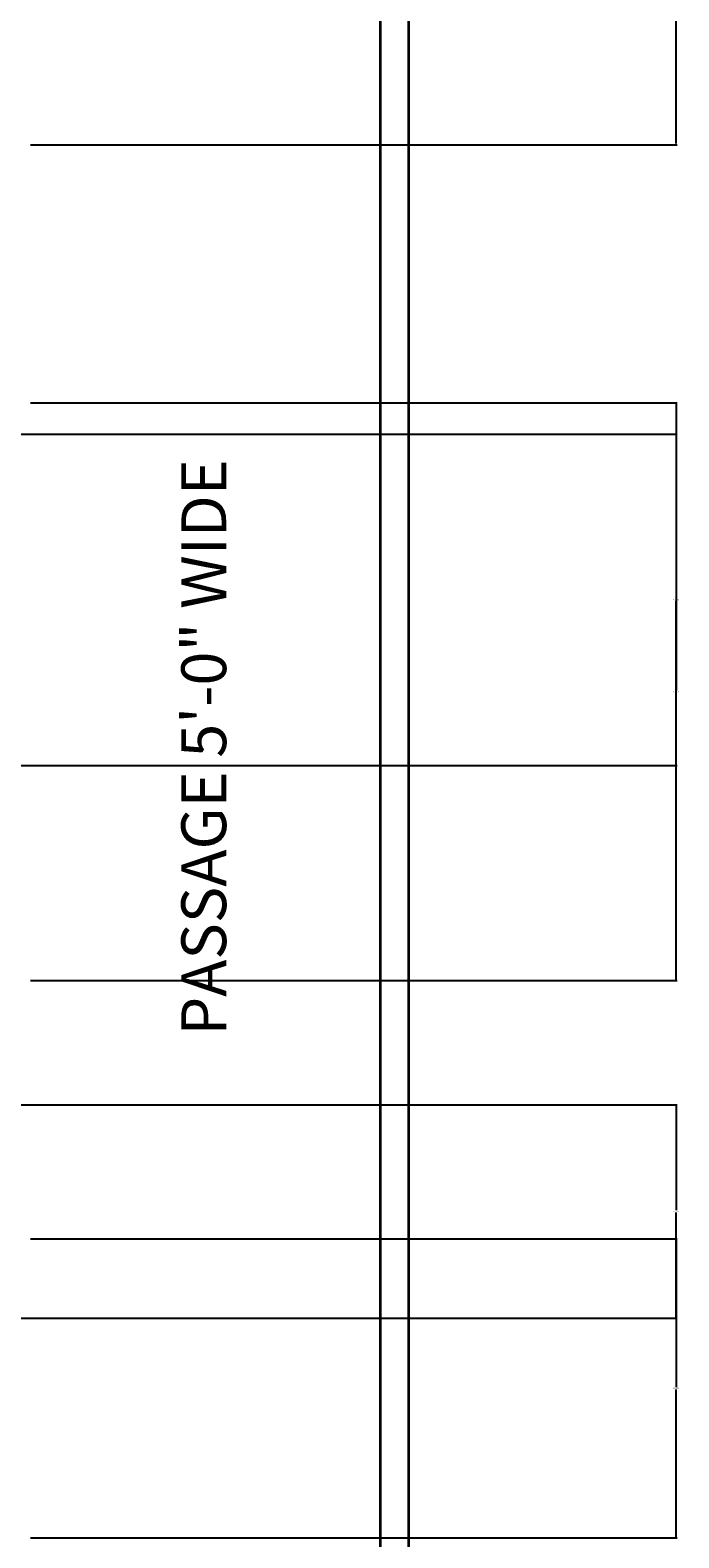
# Model space of a CAD drawing. Units: inches. Extents: x -44 to 461, y -6 to 860.
# Tile 6 of 7: x 358 to 461, y 387 to 626. Entities that reach past the tile are written whole.
import ezdxf

# ---------------------------------------------------------------- set-up
doc = ezdxf.new("R2010")
doc.units = ezdxf.units.IN
doc.header["$MEASUREMENT"] = 0
for name, color, linetype, lineweight in [('A-ANNO-DIMS', 2, 'Continuous', 18), ('A-AREA-IDEN', 7, 'Continuous', 18), ('C-PROP', 7, 'Continuous', 35)]:
    doc.layers.add(name, color=color, linetype=linetype, lineweight=lineweight)
doc.styles.get("Standard").update_dxf_attribs({"font": 'arial.ttf'})
doc.dimstyles.get("Standard").update_dxf_attribs({"dimtxt": 0.18, "dimasz": 0.18, "dimexe": 0.18, "dimexo": 0.0625, "dimgap": 0.09, "dimtad": 0, "dimtih": 1, "dimtoh": 1, "dimdec": 4, "dimzin": 0, "dimdsep": 46, "dimtxsty": 'Standard', "dimcen": 0.09, "dimadec": 0, "dimazin": 0, "dimtfac": 1, "dimtdec": 4, "dimtofl": 0, "dimtmove": 0, "dimatfit": 3, "dimfxl": 1, "dimtolj": 1, "dimtzin": 0, "dimarcsym": 0})

# ---------------------------------------------------------------- blocks, each defined once
blk = doc.blocks.new('*D51')
at = {"layer": 'A-ANNO-DIMS', "color": 0, "lineweight": -2, "transparency": 16777216}
for p, q in [((349.51, 562.18), (461.03, 562.18)), ((460.85, 562), (460.85, 536.08)), ((460.85, 509.8), (460.85, 535.72)), ((349.51, 509.62), (461.03, 509.62))]:
    blk.add_line(p, q, dxfattribs=at)
at = {"layer": 'A-ANNO-DIMS', "color": 0, "transparency": 16777216}
for points in [[(460.82, 562), (460.88, 562), (460.85, 562.18)], [(460.82, 509.8), (460.88, 509.8), (460.85, 509.62)]]:
    blk.add_solid(points, dxfattribs=at)
at = {"layer": 'Defpoints', "color": 0, "transparency": 16777216}
for p in [(349.45, 562.18), (460.85, 562.18), (349.45, 509.62)]:
    blk.add_point(p, dxfattribs=at)
at = {"layer": 'A-ANNO-DIMS', "color": 0, "transparency": 16777216, "insert": (460.85, 535.9), "char_height": 0.18, "attachment_point": 5}
blk.add_mtext('\\A1;52.5561', dxfattribs=at)
blk = doc.blocks.new('*D54')
at = {"layer": 'A-ANNO-DIMS', "color": 0, "lineweight": -2, "transparency": 16777216}
for p, q in [((342.39, 455.77), (461.03, 455.77)), ((460.85, 455.59), (460.85, 439.02)), ((460.85, 422.08), (460.85, 438.65)), ((342.39, 421.9), (461.03, 421.9))]:
    blk.add_line(p, q, dxfattribs=at)
at = {"layer": 'A-ANNO-DIMS', "color": 0, "transparency": 16777216}
for points in [[(460.82, 455.59), (460.88, 455.59), (460.85, 455.77)], [(460.82, 422.08), (460.88, 422.08), (460.85, 421.9)]]:
    blk.add_solid(points, dxfattribs=at)
at = {"layer": 'Defpoints', "color": 0, "transparency": 16777216}
for p in [(342.33, 455.77), (460.85, 455.77), (342.33, 421.9)]:
    blk.add_point(p, dxfattribs=at)
at = {"layer": 'A-ANNO-DIMS', "color": 0, "transparency": 16777216, "insert": (460.85, 438.84), "char_height": 0.18, "attachment_point": 5}
blk.add_mtext('\\A1;33.8736', dxfattribs=at)
blk = doc.blocks.new('*D60')
at = {"layer": 'A-ANNO-DIMS', "color": 0, "lineweight": -2, "transparency": 16777216}
for p, q in [((358.51, 652.02), (461.03, 652.02)), ((460.85, 651.84), (460.85, 630.26)), ((460.85, 608.32), (460.85, 629.9)), ((358.51, 608.14), (461.03, 608.14))]:
    blk.add_line(p, q, dxfattribs=at)
at = {"layer": 'A-ANNO-DIMS', "color": 0, "transparency": 16777216}
for points in [[(460.82, 651.84), (460.88, 651.84), (460.85, 652.02)], [(460.82, 608.32), (460.88, 608.32), (460.85, 608.14)]]:
    blk.add_solid(points, dxfattribs=at)
at = {"layer": 'Defpoints', "color": 0, "transparency": 16777216}
for p in [(358.45, 652.02), (358.45, 608.14), (460.85, 608.14)]:
    blk.add_point(p, dxfattribs=at)
at = {"layer": 'A-ANNO-DIMS', "color": 0, "transparency": 16777216, "insert": (460.85, 630.08), "char_height": 0.18, "attachment_point": 5}
blk.add_mtext('\\A1;43.8805', dxfattribs=at)
blk = doc.blocks.new('*D61')
at = {"layer": 'A-ANNO-DIMS', "color": 0, "lineweight": -2, "transparency": 16777216}
for p, q in [((358.51, 567.16), (461.03, 567.16)), ((460.85, 566.98), (460.85, 521.5)), ((460.85, 475.65), (460.85, 521.13)), ((358.51, 475.47), (461.03, 475.47))]:
    blk.add_line(p, q, dxfattribs=at)
at = {"layer": 'A-ANNO-DIMS', "color": 0, "transparency": 16777216}
for points in [[(460.82, 566.98), (460.88, 566.98), (460.85, 567.16)], [(460.82, 475.65), (460.88, 475.65), (460.85, 475.47)]]:
    blk.add_solid(points, dxfattribs=at)
at = {"layer": 'Defpoints', "color": 0, "transparency": 16777216}
for p in [(358.45, 567.16), (358.45, 475.47), (460.85, 475.47)]:
    blk.add_point(p, dxfattribs=at)
at = {"layer": 'A-ANNO-DIMS', "color": 0, "transparency": 16777216, "insert": (460.85, 521.31), "char_height": 0.18, "attachment_point": 5}
blk.add_mtext('\\A1;91.6879', dxfattribs=at)
blk = doc.blocks.new('*D62')
at = {"layer": 'A-ANNO-DIMS', "color": 0, "lineweight": -2, "transparency": 16777216}
for p, q in [((358.51, 434.49), (461.03, 434.49)), ((460.85, 434.31), (460.85, 410.94)), ((460.85, 387.22), (460.85, 410.58)), ((358.51, 387.04), (461.03, 387.04))]:
    blk.add_line(p, q, dxfattribs=at)
at = {"layer": 'A-ANNO-DIMS', "color": 0, "transparency": 16777216}
for points in [[(460.82, 434.31), (460.88, 434.31), (460.85, 434.49)], [(460.82, 387.22), (460.88, 387.22), (460.85, 387.04)]]:
    blk.add_solid(points, dxfattribs=at)
at = {"layer": 'Defpoints', "color": 0, "transparency": 16777216}
for p in [(358.45, 434.49), (358.45, 387.04), (460.85, 387.04)]:
    blk.add_point(p, dxfattribs=at)
at = {"layer": 'A-ANNO-DIMS', "color": 0, "transparency": 16777216, "insert": (460.85, 410.76), "char_height": 0.18, "attachment_point": 5}
blk.add_mtext('\\A1;47.4496', dxfattribs=at)

msp = doc.modelspace()

# ---------------------------------------------------------------- linework, layer by layer
at = {"layer": 'C-PROP'}
for p, q in [((418.44568, 817.0501), (418.44568, 37.0501)), ((413.94568, 752.5501), (413.94568, 262.0501))]:
    msp.add_line(p, q, dxfattribs=at)

# ---------------------------------------------------------------- texts
at = {"layer": 'A-AREA-IDEN'}
msp.add_text('PASSAGE 5\'-0" WIDE', height=7.1129656, rotation=90, dxfattribs=at).set_placement((389.52127, 466.7663))

# ---------------------------------------------------------------- dimensions: what is measured, and where the dimension line sits
at = {"layer": 'A-ANNO-DIMS'}
for base, p1, p2, picture, middle in [((460.84569, 608.14262), (358.44569, 652.02311), (358.44569, 608.14262), '*D60', (460.84569, 630.08287)), ((460.84569, 475.47002), (358.44569, 567.1579), (358.44569, 475.47002), '*D61', (460.84569, 521.31396)), ((460.84569, 562.17916), (349.44569, 509.62308), (349.44569, 562.17916), '*D51', (460.84569, 535.90112)), ((460.84569, 455.77269), (342.33163, 421.89906), (342.33163, 455.77269), '*D54', (460.84569, 438.83588)), ((460.84569, 387.03569), (358.44569, 434.4853), (358.44569, 387.03569), '*D62', (460.84569, 410.76049))]:
    dim = msp.add_linear_dim(base=base, p1=p1, p2=p2, angle=90, dimstyle='Standard', override={"dimdec": 4, "dimlfac": 1, "dimrnd": 0, "dimzin": 0, "dimdsep": 46, "dimlunit": 2}, dxfattribs=at)
    dim.commit()
    dim.dimension.update_dxf_attribs({"geometry": picture, "text_midpoint": middle})

doc.saveas('drawing.dxf')
